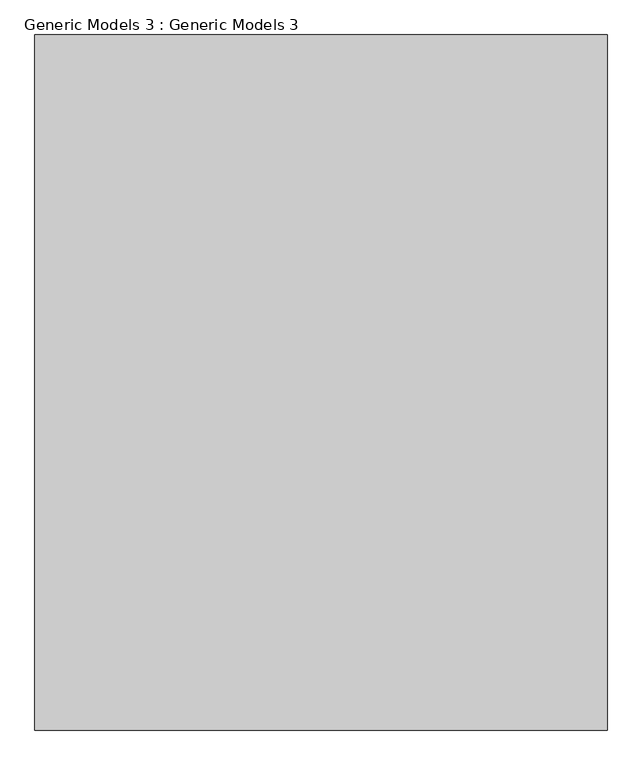
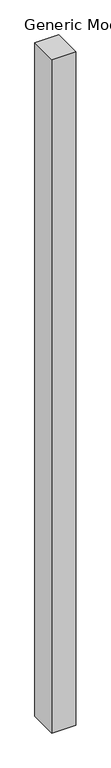
"""IFC4 building model written with IfcOpenShell, lengths in millimetres: proxy geometry, Generic Models 3 : Generic Models 3."""

from ifc_helpers import new_model, si_unit, frame, origin, place, context, project, spatial, polyline, outline, extrude, source, transform, mapped, element, save


def generic_models_3_generic_models_3_61dd9a31(model_context):
    return source(origin(), model_context, "Body", "SweptSolid", [
        extrude(outline(polyline([(-8622.8160277, -14078.0808221), (-8622.8160277, -16074.9955209), (-10267.6639665, -16074.9955209), (-10267.6639665, -14078.0808221), (-8622.8160277, -14078.0808221)])), frame((0.0, 0.0, 6629.4), z_axis=(0.0, 0.0, 1.0), x_axis=(1.0, 0.0, 0.0)), (0.0, 0.0, 1.0), 48844.2),
    ])


if __name__ == "__main__":
    model = new_model("IFC4")
    model_context = context("Model", 3, world=origin())
    ifc_project = project(units=[si_unit("LENGTHUNIT", "METRE", prefix="MILLI")], contexts=[model_context])
    site = spatial("IfcSite", under=ifc_project)
    building = spatial("IfcBuilding", under=site)
    placement = place(None, origin())
    generic_models_3_generic_models_3_shape = generic_models_3_generic_models_3_61dd9a31(model_context)
    element("IfcBuildingElementProxy", 1, Name="Generic Models 3 : Generic Models 3", ObjectType="Generic Models 3 : Generic Models 3", at=placement, inside=building, context=model_context, shape_type="MappedRepresentation", body=[
        mapped(generic_models_3_generic_models_3_shape, transform((0.0, 0.0, 0.0), x_axis=(1.0, 0.0, 0.0), y_axis=(0.0, 1.0, 0.0), z_axis=(0.0, 0.0, 1.0))),
    ])
    save(model, "model.ifc")
